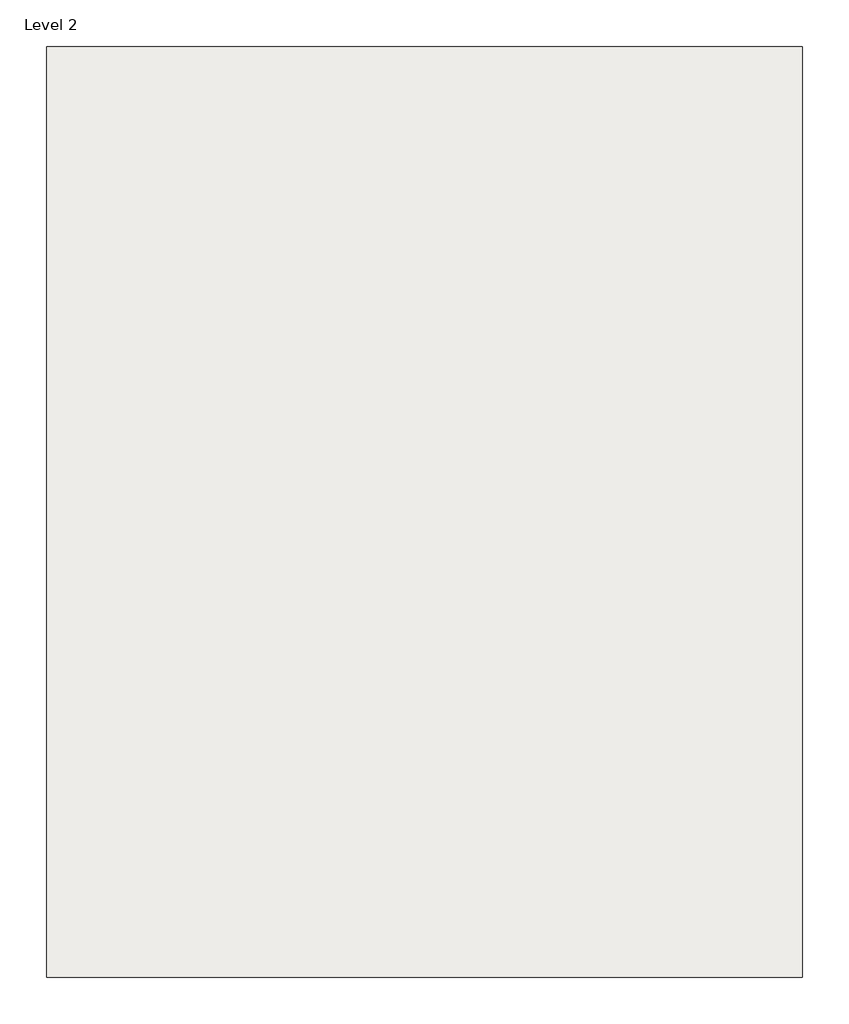
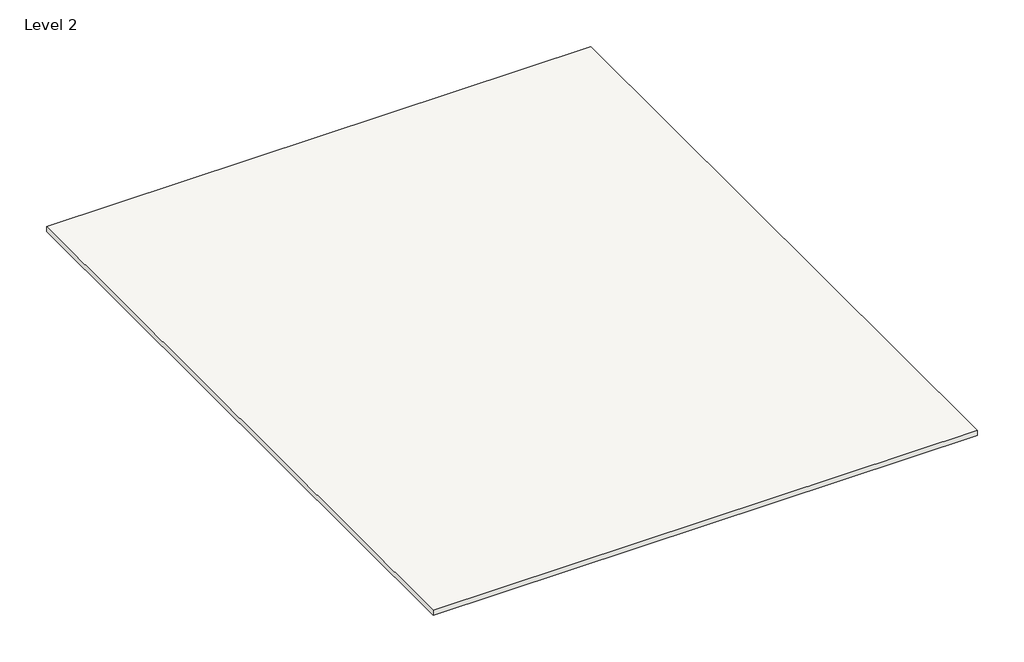
# One storey: 1 roof.
"""IFC4 building model written with IfcOpenShell, lengths in millimetres."""

from ifc_helpers import new_model, si_unit, frame, origin, place, context, project, spatial, polyline, outline, extrude, element, save

model = new_model("IFC4")

# Units and contexts
model_context = context("Model", 3, world=origin())
ifc_project = project(units=[si_unit("LENGTHUNIT", "METRE", prefix="MILLI")], contexts=[model_context])

# Site, building, storey
site = spatial("IfcSite", under=ifc_project)
building = spatial("IfcBuilding", under=site)
storey = spatial("IfcBuildingStorey", under=building, Name="Level 2", Elevation=3048.0)

# Roof
placement = place(None, origin())
element("IfcRoof", 1, ObjectType="6", at=placement, inside=storey, context=model_context, shape_type="SweptSolid", body=[
    extrude(outline(polyline([(74.1689082, 14608.7600271), (15923.7689082, 14608.7600271), (15923.7689082, -4898.4399729), (74.1689082, -4898.4399729), (74.1689082, 14608.7600271)])), frame((0.0, 0.0, 3048.0), z_axis=(0.0, 0.0, 1.0), x_axis=(1.0, 0.0, 0.0)), (0.0, 0.0, 1.0), 152.4),
])

save(model, "model.ifc")

# Revit data of these elements
# Type "6"
#   Assembly Code = "B1020"
#   Layers, outside or top first: 0' - 6" no material (function 1)
# Element 1 (IfcRoof, "6")
#   built-in parameter 1001705 = 10.5 (stored number, unit not read)
#   built-in parameter 1001710 = 33615
#   Phase Created = New Construction
#   Materials on its faces: "Default Roof"
# Materials
#   "Default Roof": colour RGB 88 101 114, transparency 0
